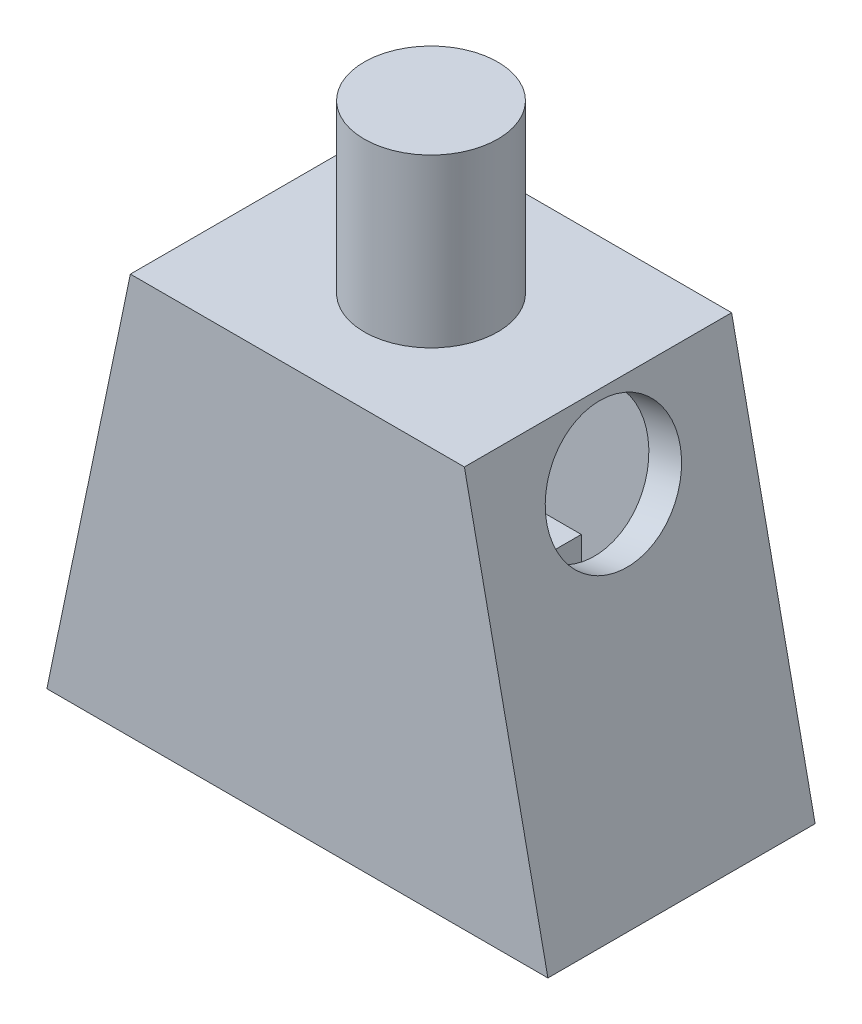
SolidWorks part; units mm, degrees
material "Plain Carbon Steel"
ref_plane "Front Plane" through (0, 0, 0) normal (0, 0, 1) x (1, 0, 0)
ref_plane "Top Plane" through (0, 0, 0) normal (0, 1, 0) x (1, 0, 0)
ref_plane "Right Plane" through (0, 0, 0) normal (1, 0, 0) x (0, 0, -1)
sketch "Torso Profile Sketch" plane through (0, 0, 0) normal (0, 0, 1) x (1, 0, 0)
  line L0 (0, 0) -> (15, 0)
  line L1 (15, 0) -> (12.5, 12)
  line L2 (12.5, 12) -> (2.5, 12)
  line L3 (2.5, 12) -> (0, 0)
  line L4 (7.5, 0) -> (7.5, 12) construction
  dimension "D1" = 15
  dimension "D2" = 10
  dimension "D3" = 12
extrude "Torso Block" add sketch "Torso Profile Sketch" against normal blind 8
shell "Torso Shell 1mm" thickness 1
sketch "Neck Stud Sketch" plane through (0, 12, 0) normal (0, 1, 0) x (1, 0, 0)
  line L0 (7.5, 8) -> (7.5, 0) construction
  line L1 (12.5, 8) -> (2.5, 8) construction
  line L2 (12.5, 0) -> (2.5, 0) construction
  circle A0 centre (7.5, 4) radius 2
  dimension "D1" = 4
extrude "Neck Stud Ø4" add sketch "Neck Stud Sketch" along normal blind 5
sketch "Arm Hole 1 Sketch" plane through (14.376, 2.995, 0) normal (0.979, 0.204, 0) x (0, 0, -1)
  line L0 (4, 9.1983) -> (4, -3.0593) construction
  line L1 (8, 9.1983) -> (0, 9.1983) construction
  line L2 (8, -3.0593) -> (0, -3.0593) construction
  circle A0 centre (4, 6.9407) radius 2
  dimension "D1" = 4
  dimension "D2" = 10
extrude "Arm Hole 1 Ø3" cut sketch "Arm Hole 1 Sketch" against normal up to next
sketch "Arm Hole 2 Sketch" plane through (0, 0, 0) normal (-0.979, 0.204, 0) x (0, 0, 1)
  line L0 (-4, 12.2577) -> (-4, 0) construction
  line L1 (-8, 12.2577) -> (0, 12.2577) construction
  line L2 (-8, 0) -> (0, 0) construction
  circle A0 centre (-4, 10) radius 2
  dimension "D1" = 4
  dimension "D2" = 10
extrude "Arm Hole 2 Ø3" cut sketch "Arm Hole 2 Sketch" against normal up to next
sketch "Hip Connector Sketch" plane through (0, 0, 0) normal (0, -1, 0) x (1, 0, 0)
  line L0 (7.5, -1) -> (7.5, -7) construction
  line L3 (6, -1) -> (6, -7)
  line L4 (9, -1) -> (9, -7)
  line L5 (1.0215, -1) -> (13.9785, -1) construction
  line L6 (6, -1) -> (9, -1)
  line L7 (1.0215, -7) -> (13.9785, -7) construction
  line L8 (6, -7) -> (9, -7)
  line L9 (6, 0) -> (6, -8) construction
  line L10 (7.5, 0) -> (7.5, -8) construction
  line L11 (9, 0) -> (9, -8) construction
  line L12 (15, -8) -> (15, 0) construction
  dimension "D3" = 6
  dimension "D1" = 1.5
  dimension "D2" = 1.5
extrude "Hip Connector Boss" add sketch "Hip Connector Sketch" against normal blind 5
